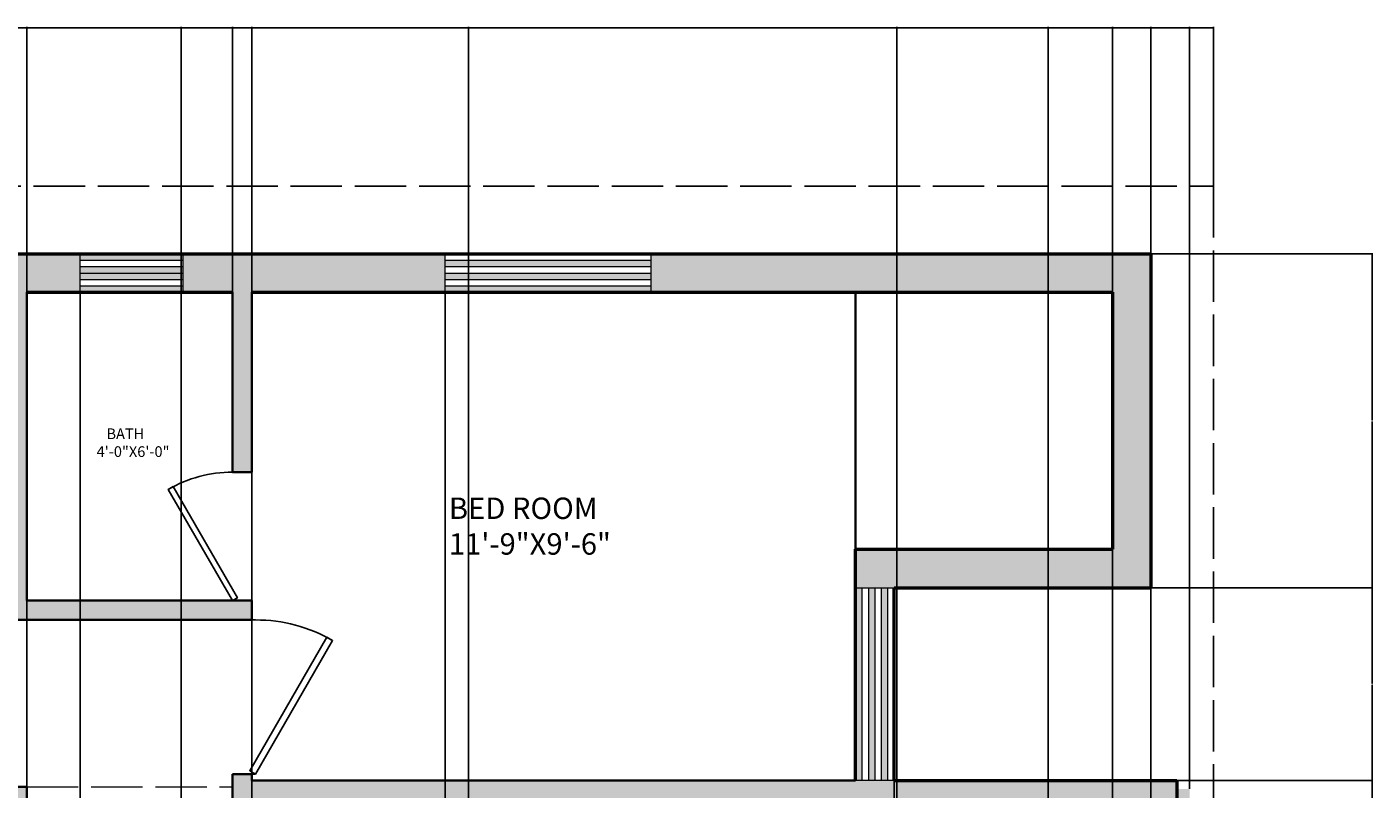
# Model space of a CAD drawing. Units: feet. Extents: x 2512 to 3087, y 1456 to 2266.
# Tile 5 of 5: x 2773 to 3087, y 2088 to 2266. Entities that reach past the tile are written whole.
import ezdxf

# ---------------------------------------------------------------- set-up
doc = ezdxf.new("R2010")
doc.units = ezdxf.units.FT
doc.linetypes.add('ACAD_ISO02W100', pattern=[15, 12, -3])
for name, color, linetype, lineweight in [('A-ANNO-DIMS', 2, 'Continuous', 18), ('A-DOOR', 240, 'Continuous', 25), ('A-GLAZ', 4, 'Continuous', 18), ('A-GLAZ-PATT', 252, 'Continuous', 13), ('A-WALL-OVHD', 8, 'ACAD_ISO02W100', 18), ('A-WALL-PATT', 252, 'Continuous', 13), ('ANNOTATION', 80, 'Continuous', 18), ('C-PROP', 8, 'ACAD_ISO02W100', 25), ('INNER WALL', 7, 'Continuous', 35), ('OPEN DOOR', 50, 'ACAD_ISO02W100', 18), ('OUTER WALL', 7, 'Continuous', 50)]:
    doc.layers.add(name, color=color, linetype=linetype, lineweight=lineweight)
doc.styles.get("Standard").update_dxf_attribs({"font": 'arial.ttf'})
doc.dimstyles.get("Standard").update_dxf_attribs({"dimtxt": 0.18, "dimasz": 0.18, "dimexe": 0.18, "dimexo": 0.0625, "dimgap": 0.09, "dimtad": 0, "dimtih": 1, "dimtoh": 1, "dimdec": 4, "dimzin": 0, "dimdsep": 46, "dimtxsty": 'Standard', "dimcen": 0.09, "dimadec": 0, "dimazin": 0, "dimtfac": 1, "dimtdec": 4, "dimtofl": 0, "dimtmove": 0, "dimatfit": 3, "dimfxl": 1, "dimtolj": 1, "dimtzin": 0, "dimarcsym": 0})

# ---------------------------------------------------------------- blocks, each defined once
blk = doc.blocks.new('*U5')
for p, q in [((0, 0), (0, -6)), ((-40, 0), (-40, -6))]:
    blk.add_line(p, q)
blk.add_lwpolyline([(0, 0), (-34.64, 20), (-35.52, 18.48), (-0.88, -1.52)], close=True)
blk.add_arc((0, 0), 40, 150, 180)
blk = doc.blocks.new('*U6')
for p, q in [((-40, 0), (-40, 6)), ((0, 0), (0, 6))]:
    blk.add_line(p, q)
blk.add_lwpolyline([(0, 0), (-34.64, -20), (-35.52, -18.48), (-0.88, 1.52)], close=True)
blk.add_arc((0, 0), 40, 180, 210)
blk = doc.blocks.new('WIN-48IN')
h = blk.add_hatch(color=256)
h.dxf.hatch_style = 1
h.paths.add_polyline_path([(0, 7.5), (0, 6), (48, 6), (48, 7.5)])
h.paths.add_polyline_path([(48, 3), (48, 4.5), (0, 4.5), (0, 3)])
h.paths.add_polyline_path([(48, 0), (48, 1.5), (0, 1.5), (0, 0)])
for p, q in [((0, 9), (48, 9)), ((0, 0), (0, 9)), ((0, 7.5), (48, 7.5)), ((48, 9), (48, 0)), ((0, 6), (48, 6)), ((0, 4.5), (48, 4.5)), ((0, 4.5), (48, 4.5)), ((0, 3), (48, 3)), ((0, 1.5), (48, 1.5)), ((48, 0), (0, 0))]:
    blk.add_line(p, q)
blk = doc.blocks.new('VENT-24IN')
h = blk.add_hatch(color=256)
h.dxf.hatch_style = 1
h.paths.add_polyline_path([(24, 7.5), (24, 9), (0, 9), (0, 7.5)])
h.paths.add_polyline_path([(0, 1.5), (0, 0), (24, 0), (24, 1.5)])
h.paths.add_polyline_path([(0, 4.5), (0, 3), (24, 3), (24, 4.5)])
h.paths.add_polyline_path([(24, 4.5), (24, 6), (0, 6), (0, 4.5)])
for p, q in [((0, 9), (24, 9)), ((0, 0), (0, 9)), ((0, 7.5), (24, 7.5)), ((24, 9), (24, 0)), ((0, 6), (24, 6)), ((0, 4.5), (24, 4.5)), ((0, 3), (24, 3)), ((0, 1.5), (24, 1.5)), ((24, 0), (0, 0))]:
    blk.add_line(p, q)
blk = doc.blocks.new('*D17')
at = {"layer": 'A-ANNO-DIMS', "color": 0, "lineweight": -2, "transparency": 16777216}
for p, q in [((2549.29, 2229.08), (2549.29, 2266.2)), ((2549.47, 2266.02), (2799.17, 2266.02)), ((3049.67, 2266.02), (2799.96, 2266.02)), ((3049.85, 2229.08), (3049.85, 2266.2))]:
    blk.add_line(p, q, dxfattribs=at)
at = {"layer": 'A-ANNO-DIMS', "color": 0, "transparency": 16777216}
for points in [[(2549.47, 2266.05), (2549.47, 2265.99), (2549.29, 2266.02)], [(3049.67, 2266.05), (3049.67, 2265.99), (3049.85, 2266.02)]]:
    blk.add_solid(points, dxfattribs=at)
at = {"layer": 'Defpoints', "color": 0, "transparency": 16777216}
for p in [(3049.85, 2266.02), (2549.29, 2229.02), (3049.85, 2229.02)]:
    blk.add_point(p, dxfattribs=at)
at = {"layer": 'A-ANNO-DIMS', "color": 0, "transparency": 16777216, "insert": (2799.57, 2266.02), "char_height": 0.18, "attachment_point": 5}
blk.add_mtext('\\A1;500.6', dxfattribs=at)
blk = doc.blocks.new('*D19')
at = {"layer": 'A-ANNO-DIMS', "color": 0, "lineweight": -2, "transparency": 16777216}
for p, q in [((2564.22, 2213.29), (2564.22, 2266.2)), ((2564.4, 2266.02), (2803.93, 2266.02)), ((3044.04, 2266.02), (2804.51, 2266.02)), ((3044.22, 2088.29), (3044.22, 2266.2))]:
    blk.add_line(p, q, dxfattribs=at)
at = {"layer": 'A-ANNO-DIMS', "color": 0, "transparency": 16777216}
for points in [[(2564.4, 2266.05), (2564.4, 2265.99), (2564.22, 2266.02)], [(3044.04, 2266.05), (3044.04, 2265.99), (3044.22, 2266.02)]]:
    blk.add_solid(points, dxfattribs=at)
at = {"layer": 'Defpoints', "color": 0, "transparency": 16777216}
for p in [(3044.22, 2266.02), (2564.22, 2213.23), (3044.22, 2088.23)]:
    blk.add_point(p, dxfattribs=at)
at = {"layer": 'A-ANNO-DIMS', "color": 0, "transparency": 16777216, "insert": (2804.22, 2266.02), "char_height": 0.18, "attachment_point": 5}
blk.add_mtext('\\A1;480', dxfattribs=at)
blk = doc.blocks.new('*D23')
at = {"layer": 'A-ANNO-DIMS', "color": 0, "lineweight": -2, "transparency": 16777216}
for p, q in [((2772.72, 2204.17), (2772.72, 1456.05)), ((2785.14, 2204.17), (2785.14, 1456.05)), ((2772.9, 1456.23), (2778.48, 1456.23)), ((2784.96, 1456.23), (2779.38, 1456.23))]:
    blk.add_line(p, q, dxfattribs=at)
at = {"layer": 'A-ANNO-DIMS', "color": 0, "transparency": 16777216}
for points in [[(2772.9, 1456.26), (2772.9, 1456.2), (2772.72, 1456.23)], [(2784.96, 1456.26), (2784.96, 1456.2), (2785.14, 1456.23)]]:
    blk.add_solid(points, dxfattribs=at)
at = {"layer": 'Defpoints', "color": 0, "transparency": 16777216}
for p in [(2772.72, 2204.23), (2785.14, 2204.23), (2785.14, 1456.23)]:
    blk.add_point(p, dxfattribs=at)
at = {"layer": 'A-ANNO-DIMS', "color": 0, "transparency": 16777216, "insert": (2778.93, 1456.23), "char_height": 0.18, "attachment_point": 5}
blk.add_mtext('\\A1;12.422', dxfattribs=at)
blk = doc.blocks.new('*D24')
at = {"layer": 'A-ANNO-DIMS', "color": 0, "lineweight": -2, "transparency": 16777216}
for p, q in [((2825.22, 2204.17), (2825.22, 1456.05)), ((2870.39, 2204.17), (2870.39, 1456.05)), ((2825.4, 1456.23), (2847.41, 1456.23)), ((2870.21, 1456.23), (2848.2, 1456.23))]:
    blk.add_line(p, q, dxfattribs=at)
at = {"layer": 'A-ANNO-DIMS', "color": 0, "transparency": 16777216}
for points in [[(2825.4, 1456.26), (2825.4, 1456.2), (2825.22, 1456.23)], [(2870.21, 1456.26), (2870.21, 1456.2), (2870.39, 1456.23)]]:
    blk.add_solid(points, dxfattribs=at)
at = {"layer": 'Defpoints', "color": 0, "transparency": 16777216}
for p in [(2825.22, 2204.23), (2870.39, 2204.23), (2870.39, 1456.23)]:
    blk.add_point(p, dxfattribs=at)
at = {"layer": 'A-ANNO-DIMS', "color": 0, "transparency": 16777216, "insert": (2847.81, 1456.23), "char_height": 0.18, "attachment_point": 5}
blk.add_mtext('\\A1;45.17', dxfattribs=at)
blk = doc.blocks.new('*D41')
at = {"layer": 'A-ANNO-DIMS', "color": 0, "lineweight": -2, "transparency": 16777216}
for p, q in [((3041.28, 2090.23), (3087.03, 2090.23)), ((3086.85, 2090.05), (3086.85, 2046.16)), ((3086.85, 2001.91), (3086.85, 2045.8)), ((3041.28, 2001.73), (3087.03, 2001.73))]:
    blk.add_line(p, q, dxfattribs=at)
at = {"layer": 'A-ANNO-DIMS', "color": 0, "transparency": 16777216}
for points in [[(3086.82, 2090.05), (3086.88, 2090.05), (3086.85, 2090.23)], [(3086.82, 2001.91), (3086.88, 2001.91), (3086.85, 2001.73)]]:
    blk.add_solid(points, dxfattribs=at)
at = {"layer": 'Defpoints', "color": 0, "transparency": 16777216}
for p in [(3041.22, 2090.23), (3086.85, 2090.23), (3041.22, 2001.73)]:
    blk.add_point(p, dxfattribs=at)
at = {"layer": 'A-ANNO-DIMS', "color": 0, "transparency": 16777216, "insert": (3086.85, 2045.98), "char_height": 0.18, "attachment_point": 5}
blk.add_mtext('\\A1;88.5', dxfattribs=at)
blk = doc.blocks.new('*D42')
at = {"layer": 'A-ANNO-DIMS', "color": 0, "lineweight": -2, "transparency": 16777216}
for p, q in [((3035.28, 2135.23), (3087.03, 2135.23)), ((3086.85, 2135.05), (3086.85, 2112.91)), ((3086.85, 2090.41), (3086.85, 2112.55)), ((3035.28, 2090.23), (3087.03, 2090.23))]:
    blk.add_line(p, q, dxfattribs=at)
at = {"layer": 'A-ANNO-DIMS', "color": 0, "transparency": 16777216}
for points in [[(3086.82, 2135.05), (3086.88, 2135.05), (3086.85, 2135.23)], [(3086.82, 2090.41), (3086.88, 2090.41), (3086.85, 2090.23)]]:
    blk.add_solid(points, dxfattribs=at)
at = {"layer": 'Defpoints', "color": 0, "transparency": 16777216}
for p in [(3035.22, 2135.23), (3086.85, 2135.23), (3035.22, 2090.23)]:
    blk.add_point(p, dxfattribs=at)
at = {"layer": 'A-ANNO-DIMS', "color": 0, "transparency": 16777216, "insert": (3086.85, 2112.73), "char_height": 0.18, "attachment_point": 5}
blk.add_mtext('\\A1;45', dxfattribs=at)
blk = doc.blocks.new('*D43')
at = {"layer": 'A-ANNO-DIMS', "color": 0, "lineweight": -2, "transparency": 16777216}
for p, q in [((3035.28, 2213.23), (3087.03, 2213.23)), ((3086.85, 2213.05), (3086.85, 2174.41)), ((3086.85, 2135.41), (3086.85, 2174.05)), ((3035.28, 2135.23), (3087.03, 2135.23))]:
    blk.add_line(p, q, dxfattribs=at)
at = {"layer": 'A-ANNO-DIMS', "color": 0, "transparency": 16777216}
for points in [[(3086.82, 2213.05), (3086.88, 2213.05), (3086.85, 2213.23)], [(3086.82, 2135.41), (3086.88, 2135.41), (3086.85, 2135.23)]]:
    blk.add_solid(points, dxfattribs=at)
at = {"layer": 'Defpoints', "color": 0, "transparency": 16777216}
for p in [(3035.22, 2213.23), (3086.85, 2213.23), (3035.22, 2135.23)]:
    blk.add_point(p, dxfattribs=at)
at = {"layer": 'A-ANNO-DIMS', "color": 0, "transparency": 16777216, "insert": (3086.85, 2174.23), "char_height": 0.18, "attachment_point": 5}
blk.add_mtext('\\A1;78', dxfattribs=at)
blk = doc.blocks.new('*D44')
at = {"layer": 'A-ANNO-DIMS', "color": 0, "lineweight": -2, "transparency": 16777216}
for p, q in [((2975.22, 2135.17), (2975.22, 1456.05)), ((3035.22, 2135.17), (3035.22, 1456.05)), ((2975.4, 1456.23), (3005, 1456.23)), ((3035.04, 1456.23), (3005.44, 1456.23))]:
    blk.add_line(p, q, dxfattribs=at)
at = {"layer": 'A-ANNO-DIMS', "color": 0, "transparency": 16777216}
for points in [[(2975.4, 1456.26), (2975.4, 1456.2), (2975.22, 1456.23)], [(3035.04, 1456.26), (3035.04, 1456.2), (3035.22, 1456.23)]]:
    blk.add_solid(points, dxfattribs=at)
at = {"layer": 'Defpoints', "color": 0, "transparency": 16777216}
for p in [(2975.22, 2135.23), (3035.22, 2135.23), (3035.22, 1456.23)]:
    blk.add_point(p, dxfattribs=at)
at = {"layer": 'A-ANNO-DIMS', "color": 0, "transparency": 16777216, "insert": (3005.22, 1456.23), "char_height": 0.18, "attachment_point": 5}
blk.add_mtext('\\A1;60', dxfattribs=at)
blk = doc.blocks.new('*D45')
at = {"layer": 'A-ANNO-DIMS', "color": 0, "lineweight": -2, "transparency": 16777216}
for p, q in [((3011.22, 1678.79), (3011.22, 2266.2)), ((3011.4, 2266.02), (3023, 2266.02)), ((3035.04, 2266.02), (3023.44, 2266.02)), ((3035.22, 1678.79), (3035.22, 2266.2))]:
    blk.add_line(p, q, dxfattribs=at)
at = {"layer": 'A-ANNO-DIMS', "color": 0, "transparency": 16777216}
for points in [[(3011.4, 2266.05), (3011.4, 2265.99), (3011.22, 2266.02)], [(3035.04, 2266.05), (3035.04, 2265.99), (3035.22, 2266.02)]]:
    blk.add_solid(points, dxfattribs=at)
at = {"layer": 'Defpoints', "color": 0, "transparency": 16777216}
for p in [(3035.22, 2266.02), (3011.22, 1678.73), (3035.22, 1678.73)]:
    blk.add_point(p, dxfattribs=at)
at = {"layer": 'A-ANNO-DIMS', "color": 0, "transparency": 16777216, "insert": (3023.22, 2266.02), "char_height": 0.18, "attachment_point": 5}
blk.add_mtext('\\A1;24', dxfattribs=at)
blk = doc.blocks.new('*D50')
at = {"layer": 'A-ANNO-DIMS', "color": 0, "lineweight": -2, "transparency": 16777216}
for p, q in [((2875.84, 1903.79), (2875.84, 2266.2)), ((2876.02, 2266.02), (2925.56, 2266.02)), ((2975.66, 2266.02), (2926.12, 2266.02)), ((2975.84, 1903.79), (2975.84, 2266.2))]:
    blk.add_line(p, q, dxfattribs=at)
at = {"layer": 'A-ANNO-DIMS', "color": 0, "transparency": 16777216}
for points in [[(2876.02, 2266.05), (2876.02, 2265.99), (2875.84, 2266.02)], [(2975.66, 2266.05), (2975.66, 2265.99), (2975.84, 2266.02)]]:
    blk.add_solid(points, dxfattribs=at)
at = {"layer": 'Defpoints', "color": 0, "transparency": 16777216}
for p in [(2975.84, 2266.02), (2875.84, 1903.73), (2975.84, 1903.73)]:
    blk.add_point(p, dxfattribs=at)
at = {"layer": 'A-ANNO-DIMS', "color": 0, "transparency": 16777216, "insert": (2925.84, 2266.02), "char_height": 0.18, "attachment_point": 5}
blk.add_mtext('\\A1;100', dxfattribs=at)
blk = doc.blocks.new('*D51')
at = {"layer": 'A-ANNO-DIMS', "color": 0, "lineweight": -2, "transparency": 16777216}
for p, q in [((2975.84, 1903.79), (2975.84, 2266.2)), ((2976.02, 2266.02), (3000.63, 2266.02)), ((3026.04, 2266.02), (3001.42, 2266.02)), ((3026.22, 1903.79), (3026.22, 2266.2))]:
    blk.add_line(p, q, dxfattribs=at)
at = {"layer": 'A-ANNO-DIMS', "color": 0, "transparency": 16777216}
for points in [[(2976.02, 2266.05), (2976.02, 2265.99), (2975.84, 2266.02)], [(3026.04, 2266.05), (3026.04, 2265.99), (3026.22, 2266.02)]]:
    blk.add_solid(points, dxfattribs=at)
at = {"layer": 'Defpoints', "color": 0, "transparency": 16777216}
for p in [(3026.22, 2266.02), (2975.84, 1903.73), (3026.22, 1903.73)]:
    blk.add_point(p, dxfattribs=at)
at = {"layer": 'A-ANNO-DIMS', "color": 0, "transparency": 16777216, "insert": (3001.03, 2266.02), "char_height": 0.18, "attachment_point": 5}
blk.add_mtext('\\A1;50.38', dxfattribs=at)
blk = doc.blocks.new('*D52')
at = {"layer": 'A-ANNO-DIMS', "color": 0, "lineweight": -2, "transparency": 16777216}
for p, q in [((2772.72, 1813.15), (2772.72, 2266.2)), ((2772.9, 2266.02), (2790.5, 2266.02)), ((2808.54, 2266.02), (2790.94, 2266.02)), ((2808.72, 1816.79), (2808.72, 2266.2))]:
    blk.add_line(p, q, dxfattribs=at)
at = {"layer": 'A-ANNO-DIMS', "color": 0, "transparency": 16777216}
for points in [[(2772.9, 2266.05), (2772.9, 2265.99), (2772.72, 2266.02)], [(2808.54, 2266.05), (2808.54, 2265.99), (2808.72, 2266.02)]]:
    blk.add_solid(points, dxfattribs=at)
at = {"layer": 'Defpoints', "color": 0, "transparency": 16777216}
for p in [(2808.72, 2266.02), (2808.72, 1816.73), (2772.72, 1813.09)]:
    blk.add_point(p, dxfattribs=at)
at = {"layer": 'A-ANNO-DIMS', "color": 0, "transparency": 16777216, "insert": (2790.72, 2266.02), "char_height": 0.18, "attachment_point": 5}
blk.add_mtext('\\A1;36', dxfattribs=at)
blk = doc.blocks.new('*D54')
at = {"layer": 'A-ANNO-DIMS', "color": 0, "lineweight": -2, "transparency": 16777216}
for p, q in [((2772.72, 2132.17), (2772.72, 1456.05)), ((2763.72, 2127.67), (2763.72, 1456.05)), ((2763.9, 1456.23), (2768.07, 1456.23)), ((2772.54, 1456.23), (2768.37, 1456.23))]:
    blk.add_line(p, q, dxfattribs=at)
at = {"layer": 'A-ANNO-DIMS', "color": 0, "transparency": 16777216}
for points in [[(2763.9, 1456.26), (2763.9, 1456.2), (2763.72, 1456.23)], [(2772.54, 1456.26), (2772.54, 1456.2), (2772.72, 1456.23)]]:
    blk.add_solid(points, dxfattribs=at)
at = {"layer": 'Defpoints', "color": 0, "transparency": 16777216}
for p in [(2772.72, 2132.23), (2763.72, 2127.73), (2772.72, 1456.23)]:
    blk.add_point(p, dxfattribs=at)
at = {"layer": 'A-ANNO-DIMS', "color": 0, "transparency": 16777216, "insert": (2768.22, 1456.23), "char_height": 0.18, "attachment_point": 5}
blk.add_mtext('\\A1;9', dxfattribs=at)
blk = doc.blocks.new('*D55')
at = {"layer": 'A-ANNO-DIMS', "color": 0, "lineweight": -2, "transparency": 16777216}
for p, q in [((2820.72, 2162.29), (2820.72, 2266.2)), ((2820.9, 2266.02), (2822.71, 2266.02)), ((2825.04, 2266.02), (2823.23, 2266.02)), ((2825.22, 2162.29), (2825.22, 2266.2))]:
    blk.add_line(p, q, dxfattribs=at)
at = {"layer": 'A-ANNO-DIMS', "color": 0, "transparency": 16777216}
for points in [[(2820.9, 2266.05), (2820.9, 2265.99), (2820.72, 2266.02)], [(2825.04, 2266.05), (2825.04, 2265.99), (2825.22, 2266.02)]]:
    blk.add_solid(points, dxfattribs=at)
at = {"layer": 'Defpoints', "color": 0, "transparency": 16777216}
for p in [(2825.22, 2266.02), (2820.72, 2162.23), (2825.22, 2162.23)]:
    blk.add_point(p, dxfattribs=at)
at = {"layer": 'A-ANNO-DIMS', "color": 0, "transparency": 16777216, "insert": (2822.97, 2266.02), "char_height": 0.18, "attachment_point": 5}
blk.add_mtext('\\A1;4.5', dxfattribs=at)

msp = doc.modelspace()

# ---------------------------------------------------------------- hatches: boundary and pattern name
at = {"layer": 'A-GLAZ-PATT'}
h = msp.add_hatch(color=256, dxfattribs=at)
h.dxf.hatch_style = 1
h.paths.add_polyline_path([(2969.2185, 2090.2254), (2970.7185, 2090.2254), (2970.7185, 2135.213), (2969.2185, 2135.213)])
h.paths.add_polyline_path([(2972.2185, 2090.2254), (2973.7185, 2090.2254), (2973.7185, 2135.213), (2972.2185, 2135.213)])
h.paths.add_polyline_path([(2966.2185, 2090.2254), (2967.7185, 2090.2254), (2967.7185, 2135.213), (2966.2185, 2135.213)])
at = {"layer": 'A-WALL-PATT'}
h = msp.add_hatch(color=256, dxfattribs=at)
h.dxf.hatch_style = 1
h.paths.add_polyline_path([(3035.2185, 1915.2872), (3026.2185, 1915.2872), (3026.2185, 1912.7316), (2936.2185, 1912.7316), (2936.2185, 2001.7316), (2931.7185, 2001.7316), (2931.7185, 1912.7316), (2808.7185, 1912.7316), (2808.7185, 1903.7316), (3026.2185, 1903.7316), (3026.2185, 1816.7316), (2808.7185, 1816.7316), (2808.7185, 1807.7316), (2823.7185, 1807.7316), (2823.7185, 1638.2316), (2828.2185, 1638.2316), (2828.2185, 1674.2316), (2828.2185, 1678.7316), (2828.2185, 1807.7316), (3026.2185, 1807.7316), (3026.2185, 1735.7316), (3002.2185, 1735.7316), (3002.2546, 1726.7316), (3011.2546, 1726.7316), (3035.2185, 1726.7316)])
h.paths.add_polyline_path([(3035.2185, 2001.7316), (2990.2185, 2001.7316), (2972.2185, 2001.7316), (2972.2185, 1996.7316), (3026.2185, 1996.7316), (3026.2185, 1963.2872), (3035.2185, 1963.2872)], flags=17)
h.paths.add_polyline_path([(3041.2185, 2010.7316), (2990.2185, 2010.7316), (2990.2185, 2001.7316), (3035.2185, 2001.7316), (3041.2185, 2001.7316)])
h.paths.add_polyline_path([(3044.2185, 2085.7316), (3044.2185, 2088.2316), (3041.2185, 2088.2316), (3041.2185, 2006.2316), (3044.2185, 2006.2316)])
h.paths.add_polyline_path([(3041.2185, 2090.2316), (2975.2185, 2090.2316), (2975.2185, 2090.2254), (2966.2185, 2090.2254), (2825.2185, 2090.2316), (2825.2185, 2091.7316), (2820.7185, 2091.7316), (2820.7185, 2085.7316), (2820.7185, 2084.2316), (2825.2185, 2084.2316), (2825.2185, 2085.7316), (2990.2185, 2085.7316), (2990.2185, 2046.7316), (2999.2185, 2046.7316), (2999.2185, 2085.7316), (3041.2185, 2085.7316)])
h.paths.add_polyline_path([(3035.2185, 2213.2316), (2918.3922, 2213.2316), (2918.3922, 2204.2316), (3026.2185, 2204.2316), (3026.2185, 2144.2316), (2966.2185, 2144.2316), (2966.2185, 2135.213), (2975.2185, 2135.213), (2975.2185, 2135.2316), (3035.2185, 2135.2316)])
h.paths.add_polyline_path([(2870.3922, 2213.2316), (2809.1404, 2213.2316), (2809.1404, 2204.2316), (2820.7185, 2204.2316), (2820.7185, 2162.2316), (2825.2185, 2162.2316), (2825.2185, 2204.2316), (2870.3922, 2204.2316)])
h.paths.add_polyline_path([(2785.1404, 2213.2316), (2751.447, 2213.2316), (2751.447, 2204.2316), (2763.7185, 2204.2316), (2763.7185, 2127.7316), (2825.2185, 2127.7316), (2825.2185, 2132.2316), (2820.7185, 2132.2316), (2772.7185, 2132.2316), (2772.7185, 2204.2316), (2785.1404, 2204.2316)])
h.paths.add_polyline_path([(2727.447, 2213.2316), (2656.8898, 2213.2316), (2656.8898, 2204.2316), (2711.2185, 2204.2316), (2711.2185, 2124.7316), (2715.7185, 2124.7316), (2715.7185, 2127.7316), (2733.7185, 2127.7316), (2733.7185, 2132.2316), (2715.7185, 2132.2316), (2715.7185, 2204.2316), (2727.447, 2204.2316)], flags=17)
h.paths.add_polyline_path([(2608.8898, 2213.2316), (2564.2185, 2213.2316), (2564.2185, 2079.7316), (2609.2185, 2079.7316), (2609.2185, 2037.7316), (2618.2185, 2037.7316), (2618.2185, 2079.7316), (2763.7185, 2079.7316), (2763.7185, 2007.7316), (2654.2185, 2007.7316), (2654.2185, 2003.2316), (2763.7185, 2003.2316), (2763.7185, 1891.0755), (2772.7185, 1891.0234), (2772.7185, 1903.7316), (2772.7185, 2088.7316), (2573.2185, 2088.7316), (2573.2185, 2204.2316), (2608.8898, 2204.2316)])
h.paths.add_polyline_path([(2567.2185, 2079.7316), (2564.2185, 2079.7316), (2564.2185, 2007.7316), (2567.2185, 2007.7316)], flags=17)
h.paths.add_polyline_path([(2618.2185, 2007.7316), (2564.2185, 2007.7316), (2564.2185, 2003.2171), (2573.2185, 2003.2171), (2573.2185, 2003.2316), (2618.2185, 2003.2316)], flags=17)
h.paths.add_polyline_path([(2573.2185, 1955.2171), (2564.2185, 1955.2171), (2564.2185, 1904.096), (2573.2185, 1904.096)], flags=17)
h.paths.add_polyline_path([(2573.2185, 1851.677), (2603.2185, 1851.5035), (2603.2195, 1856.0035), (2573.2185, 1856.1771), (2573.2185, 1856.096), (2564.2185, 1856.096), (2564.2185, 1785.728), (2594.2185, 1785.5544), (2600.2185, 1785.5197), (2637.7185, 1785.3028), (2637.7185, 1855.8039), (2633.2185, 1855.83), (2633.2185, 1789.8289), (2573.2185, 1790.176)])
h.paths.add_polyline_path([(2772.7185, 1855.0228), (2767.3185, 1855.0228), (2767.3004, 1855.0542), (2673.7185, 1855.5956), (2673.7185, 1851.0956), (2763.7185, 1850.575), (2763.7185, 1743.5732), (2564.2185, 1744.7273), (2564.2185, 1719.3702), (2573.2185, 1719.3702), (2573.2185, 1735.6751), (2633.2185, 1735.328), (2633.2185, 1717.3272), (2637.7185, 1717.3272), (2637.7185, 1735.302), (2772.7185, 1734.521)])
h.paths.add_polyline_path([(2697.7185, 1734.9549), (2693.2185, 1734.9809), (2693.2185, 1602.8011), (2697.7185, 1602.8011)])
h.paths.add_polyline_path([(2823.7185, 1561.2231), (2733.7185, 1561.7437), (2733.7185, 1552.7436), (2823.7185, 1552.2229)])
h.paths.add_polyline_path([(2697.7185, 1566.8011), (2693.2185, 1566.8011), (2693.2185, 1562.8011), (2682.4194, 1562.8011), (2682.4194, 1553.8011), (2693.2185, 1553.8011), (2693.2185, 1495.2316), (2697.7185, 1495.2316)])
h.paths.add_polyline_path([(2828.2185, 1495.2316), (2693.2185, 1495.2316), (2693.2185, 1493.2316), (2828.2185, 1493.2316)])
h.paths.add_polyline_path([(2828.2185, 1602.2316), (2823.7185, 1602.2316), (2823.7185, 1495.2316), (2828.2185, 1495.2316)])
h.paths.add_polyline_path([(3035.2185, 1523.0765), (3026.2185, 1523.0765), (3026.2185, 1513.7316), (2828.2185, 1513.7316), (2828.2185, 1504.7316), (3035.2185, 1504.7316)])
h.paths.add_polyline_path([(3026.2185, 1602.2316), (2906.2185, 1602.2316), (2906.2185, 1644.2316), (2901.7185, 1644.2316), (2901.7185, 1597.7316), (3026.2185, 1597.7316)])
h.paths.add_polyline_path([(3035.2185, 1678.7316), (2864.2185, 1678.7316), (2864.2185, 1674.2316), (3026.2185, 1674.2316), (3026.2185, 1642.5123), (3035.2185, 1642.5123)], flags=17)
h.paths.add_polyline_path([(3035.2185, 1618.5123), (3026.2185, 1618.5123), (3026.2185, 1571.0765), (3035.2185, 1571.0765)])
h = msp.add_hatch(color=256, dxfattribs=at)
h.dxf.hatch_style = 1
h.paths.add_polyline_path([(2573.2185, 2204.2316), (2608.8898, 2204.2316), (2608.8898, 2213.2316), (2564.2185, 2213.2316), (2564.2185, 2079.7316), (2609.2185, 2079.7316), (2609.2185, 2037.7316), (2613.7185, 2037.7316), (2618.2185, 2037.7316), (2618.2185, 2079.7316), (2763.7185, 2079.7316), (2763.7185, 2007.7316), (2654.2185, 2007.7316), (2654.2185, 2003.2316), (2763.7185, 2003.2316), (2763.7185, 1891.0755), (2772.7185, 1891.0234), (2772.7185, 1903.7316), (2772.7185, 2088.7316), (2573.2185, 2088.7316)])
h.paths.add_polyline_path([(2727.447, 2213.2316), (2656.8898, 2213.2316), (2656.8898, 2204.2316), (2711.2185, 2204.2316), (2711.2185, 2124.7316), (2715.7185, 2124.7316), (2715.7185, 2127.7316), (2733.7185, 2127.7316), (2733.7185, 2132.2316), (2715.7185, 2132.2316), (2715.7185, 2204.2316), (2727.447, 2204.2316)], flags=17)
h.paths.add_polyline_path([(2785.1404, 2213.2316), (2751.447, 2213.2316), (2751.447, 2204.2316), (2763.7185, 2204.2316), (2763.7185, 2127.7316), (2825.2185, 2127.7316), (2825.2185, 2132.2316), (2820.7185, 2132.2316), (2772.7185, 2132.2316), (2772.7185, 2204.2316), (2785.1404, 2204.2316)])
h.paths.add_polyline_path([(2966.2185, 2204.2316), (2825.2185, 2204.2316), (2825.2185, 2162.2316), (2820.7185, 2162.2316, 0.12053744), (2806.8695, 2158.8438), (2822.234, 2132.2316), (2825.2185, 2132.2316), (2825.2185, 2127.7316), (2826.1185, 2127.7316, -0.12053744), (2842.7373, 2123.6662), (2842.7545, 2123.696), (2844.1185, 2122.9085), (2826.1185, 2091.7316), (2825.2185, 2091.7316), (2825.2185, 2090.2316), (2966.2185, 2090.2316), (2966.2185, 2135.213), (2966.2185, 2144.2316)], flags=17)
h.paths.add_polyline_path([(2870.3922, 2213.2316), (2809.1404, 2213.2316), (2809.1404, 2204.2316), (2820.7185, 2204.2316), (2820.7185, 2162.2316), (2825.2185, 2162.2316), (2825.2185, 2204.2316), (2870.3922, 2204.2316)])
h.paths.add_polyline_path([(3035.2185, 2213.2316), (2918.3922, 2213.2316), (2918.3922, 2204.2316), (3026.2185, 2204.2316), (3026.2185, 2144.2316), (2966.2185, 2144.2316), (2966.2185, 2135.213), (2975.2185, 2135.213), (2975.2185, 2135.2316), (3035.2185, 2135.2316)])
h.paths.add_polyline_path([(2999.2185, 2085.7316), (3041.2185, 2085.7316), (3041.2185, 2090.2316), (2975.2185, 2090.2316), (2975.2185, 2090.2254), (2966.2185, 2090.2254), (2825.2185, 2090.2316), (2825.2185, 2091.7316), (2820.7185, 2091.7316), (2820.7185, 2085.7316), (2820.7185, 2084.2316), (2825.2185, 2084.2316), (2825.2185, 2085.7316), (2990.2185, 2085.7316), (2990.2185, 2046.7316), (2995.6185, 2046.7316), (2999.2185, 2046.7316)])
h.paths.add_polyline_path([(3041.2185, 2010.7316), (2990.2185, 2010.7316), (2990.2185, 2001.7316), (3041.2185, 2001.7316)])
h.paths.add_polyline_path([(3035.2185, 2001.7316), (2990.2185, 2001.7316), (2972.2185, 2001.7316), (2972.2185, 1996.7316), (3026.2185, 1996.7316), (3026.2185, 1963.2872), (3035.2185, 1963.2872)])
h.paths.add_polyline_path([(3044.2185, 2085.7316), (3044.2185, 2088.2316), (3041.2185, 2088.2316), (3041.2185, 2085.7316), (3041.2185, 2006.2316), (3044.2185, 2006.2316)])
h.paths.add_polyline_path([(2966.2185, 2135.213), (2966.2185, 2144.2316), (2966.2185, 2204.2316), (2918.3922, 2204.2316), (2825.2185, 2204.2316), (2825.2185, 2162.2316), (2820.7185, 2162.2316, 0.12053744), (2806.8695, 2158.8438), (2822.234, 2132.2316), (2825.2185, 2132.2316), (2825.2185, 2127.7316), (2826.1185, 2127.7316, -0.12053744), (2842.7373, 2123.6662), (2842.7545, 2123.696), (2844.1185, 2122.9085), (2826.1185, 2091.7316), (2825.2185, 2091.7316), (2825.2185, 2090.2316), (2966.2185, 2090.2316)], flags=17)
h.paths.add_polyline_path([(2869.2463, 2140.1407), (2910.0273, 2140.1407), (2910.0273, 2158.8321), (2869.2463, 2158.8321)], flags=8)

# ---------------------------------------------------------------- linework, layer by layer
at = {"layer": 'A-GLAZ'}
for p, q in [((2966.2185, 2090.2254), (2966.2185, 2135.213)), ((2966.2185, 2135.213), (2975.2185, 2135.213)), ((2967.7185, 2135.213), (2967.7185, 2090.2254)), ((2969.2185, 2135.213), (2969.2185, 2090.2254)), ((2970.7185, 2135.213), (2970.7185, 2090.2254)), ((2970.7185, 2135.213), (2970.7185, 2090.2254)), ((2972.2185, 2135.213), (2972.2185, 2090.2254)), ((2973.7185, 2135.213), (2973.7185, 2090.2254)), ((2975.2185, 2135.213), (2975.2185, 2090.2254)), ((2975.2185, 2090.2254), (2966.2185, 2090.2254))]:
    msp.add_line(p, q, dxfattribs=at)
at = {"layer": 'A-WALL-OVHD'}
msp.add_line((3035.2185, 2135.2316), (3035.2185, 2090.2316), dxfattribs=at)
at = {"layer": 'C-PROP'}
for p, q in [((2549.289, 2229.0217), (3049.8469, 2229.0217)), ((3049.8469, 2229.0217), (3049.8469, 1493.2316))]:
    msp.add_line(p, q, dxfattribs=at)
at = {"layer": 'INNER WALL'}
for p, q in [((2772.7185, 2132.2316), (2772.7185, 2204.2316)), ((2820.7185, 2162.2316), (2820.7185, 2204.2316)), ((2825.2185, 2162.2316), (2825.2185, 2204.2316)), ((2966.2185, 2144.2316), (2966.2185, 2204.2316)), ((2820.7185, 2162.2316), (2825.2185, 2162.2316)), ((2772.7185, 2132.2316), (2825.2185, 2132.2316)), ((2825.2185, 2127.7316), (2825.2185, 2132.2316)), ((2763.7185, 2127.7316), (2825.2185, 2127.7316)), ((2820.7185, 2085.7316), (2820.7185, 2091.7316)), ((2820.7185, 2091.7316), (2825.2185, 2091.7316)), ((2825.2185, 2090.2316), (2825.2185, 2091.7316)), ((2573.2185, 2088.7316), (2772.7185, 2088.7316)), ((2772.7185, 2088.7316), (2772.7185, 1903.7316)), ((2825.2185, 2090.2316), (2966.2185, 2090.2316))]:
    msp.add_line(p, q, dxfattribs=at)
at = {"layer": 'OPEN DOOR'}
msp.add_line((2772.7185, 2088.7316), (2820.7185, 2088.7316), dxfattribs=at)
at = {"layer": 'OUTER WALL'}
for p, q in [((2564.2185, 2213.2316), (3035.2185, 2213.2316)), ((3035.2185, 2213.2316), (3035.2185, 2135.2316)), ((2772.7185, 2204.2316), (2820.7185, 2204.2316)), ((2825.2185, 2204.2316), (3026.2185, 2204.2316)), ((3026.2185, 2204.2316), (3026.2185, 2144.2316)), ((2966.2185, 2090.2316), (2966.2185, 2144.2316)), ((2966.2185, 2144.2316), (3026.2185, 2144.2316)), ((2975.2185, 2135.2316), (3035.2185, 2135.2316)), ((2975.2185, 2090.2316), (2975.2185, 2135.2316)), ((2975.2185, 2090.2316), (3041.2185, 2090.2316)), ((3041.2185, 2090.2316), (3041.2185, 2001.7316))]:
    msp.add_line(p, q, dxfattribs=at)

# ---------------------------------------------------------------- block references
at = {"layer": 'A-DOOR', "rotation": 270}
for name, p, xscale, yscale, zscale in [('*U6', (2820.7185, 2132.2316), 0.7500000000000038, 0.7500000000000038, 0.7500000000000038), ('*U5', (2826.1185, 2091.7316), 0.899999999999959, 0.899999999999959, 0.899999999999959)]:
    msp.add_blockref(name, p, dxfattribs=dict(at, xscale=xscale, yscale=yscale, zscale=zscale))
at = {"layer": 'A-GLAZ'}
for name, p in [('VENT-24IN', (2785.1404, 2204.232)), ('WIN-48IN', (2870.3924, 2204.232))]:
    msp.add_blockref(name, p, dxfattribs=at)

# ---------------------------------------------------------------- texts
at = {"layer": 'ANNOTATION', "attachment_point": 1}
for s, width, insert, char_height in [('   BATH\\P4\'-0"X6\'-0"', 16.842597, (2788.9935, 2172.4527), 2.5), ('\\A1;BED ROOM\\P11\'-9"X9\'-6"', 38.558323, (2871.2569, 2156.3031), 5)]:
    msp.add_mtext_dynamic_manual_height_columns(s, width=width, gutter_width=12.5, heights=[0], dxfattribs=dict(at, insert=insert, char_height=char_height))

# ---------------------------------------------------------------- dimensions: what is measured, and where the dimension line sits
at = {"layer": 'A-ANNO-DIMS'}
for base, p1, p2, override, picture, middle in [((3049.8469, 2266.0217), (2549.289, 2229.0217), (3049.8469, 2229.0217), {"dimdec": 1, "dimlfac": 1, "dimrnd": 0, "dimzin": 0, "dimdsep": 46, "dimlunit": 2}, '*D17', (2799.5679, 2266.0217)), ((3044.2185, 2266.0217), (2564.2185, 2213.2316), (3044.2185, 2088.2316), {"dimdec": 0, "dimlfac": 1, "dimrnd": 0, "dimzin": 0, "dimdsep": 46, "dimlunit": 2}, '*D19', (2804.2185, 2266.0217)), ((2808.7185, 2266.0217), (2772.7185, 1813.092), (2808.7185, 1816.7316), {"dimdec": 0, "dimlfac": 1, "dimrnd": 0, "dimzin": 0, "dimdsep": 46, "dimlunit": 2}, '*D52', (2790.7185, 2266.0217)), ((2825.2185, 2266.0217), (2820.7185, 2162.2316), (2825.2185, 2162.2316), {"dimdec": 1, "dimlfac": 1, "dimrnd": 0, "dimzin": 0, "dimdsep": 46, "dimlunit": 2}, '*D55', (2822.9685, 2266.0217)), ((2975.8387, 2266.0217), (2875.8387, 1903.7316), (2975.8387, 1903.7316), {"dimdec": 0, "dimlfac": 1, "dimrnd": 0, "dimzin": 0, "dimdsep": 46, "dimlunit": 2}, '*D50', (2925.8387, 2266.0217)), ((3026.2185, 2266.0217), (2975.8387, 1903.7316), (3026.2185, 1903.7316), {"dimdec": 2, "dimlfac": 1, "dimrnd": 0, "dimzin": 0, "dimdsep": 46, "dimlunit": 2}, '*D51', (3001.0286, 2266.0217)), ((3035.2185, 2266.0217), (3011.2185, 1678.7316), (3035.2185, 1678.7316), {"dimdec": 0, "dimlfac": 1, "dimrnd": 0, "dimzin": 0, "dimdsep": 46, "dimlunit": 2}, '*D45', (3023.2185, 2266.0217)), ((2785.1404, 1456.2316), (2772.7185, 2204.2316), (2785.1404, 2204.2316), {"dimdec": 3, "dimlfac": 1, "dimrnd": 0, "dimzin": 0, "dimdsep": 46, "dimlunit": 2}, '*D23', (2778.9294, 1456.2316)), ((2870.3922, 1456.2316), (2825.2185, 2204.2316), (2870.3922, 2204.2316), {"dimdec": 2, "dimlfac": 1, "dimrnd": 0, "dimzin": 0, "dimdsep": 46, "dimlunit": 2}, '*D24', (2847.8054, 1456.2316)), ((3035.2185, 1456.2316), (2975.2185, 2135.2316), (3035.2185, 2135.2316), {"dimdec": 0, "dimlfac": 1, "dimrnd": 0, "dimzin": 0, "dimdsep": 46, "dimlunit": 2}, '*D44', (3005.2185, 1456.2316)), ((2772.7185, 1456.2316), (2763.7185, 2127.7316), (2772.7185, 2132.2316), {"dimdec": 0, "dimlfac": 1, "dimrnd": 0, "dimzin": 0, "dimdsep": 46, "dimlunit": 2}, '*D54', (2768.2185, 1456.2316))]:
    dim = msp.add_linear_dim(base=base, p1=p1, p2=p2, dimstyle='Standard', override=override, dxfattribs=at)
    dim.commit()
    dim.dimension.update_dxf_attribs({"geometry": picture, "text_midpoint": middle})
for base, p1, p2, override, picture, middle in [((3086.8469, 2213.2316), (3035.2185, 2135.2316), (3035.2185, 2213.2316), {"dimdec": 0, "dimlfac": 1, "dimrnd": 0, "dimzin": 0, "dimdsep": 46, "dimlunit": 2}, '*D43', (3086.8469, 2174.2316)), ((3086.8469, 2135.2316), (3035.2185, 2090.2316), (3035.2185, 2135.2316), {"dimdec": 0, "dimlfac": 1, "dimrnd": 0, "dimzin": 0, "dimdsep": 46, "dimlunit": 2}, '*D42', (3086.8469, 2112.7316)), ((3086.8469, 2090.2316), (3041.2185, 2001.7316), (3041.2185, 2090.2316), {"dimdec": 1, "dimlfac": 1, "dimrnd": 0, "dimzin": 0, "dimdsep": 46, "dimlunit": 2}, '*D41', (3086.8469, 2045.9816))]:
    dim = msp.add_linear_dim(base=base, p1=p1, p2=p2, angle=90, dimstyle='Standard', override=override, dxfattribs=at)
    dim.commit()
    dim.dimension.update_dxf_attribs({"geometry": picture, "text_midpoint": middle})

doc.saveas('drawing.dxf')
